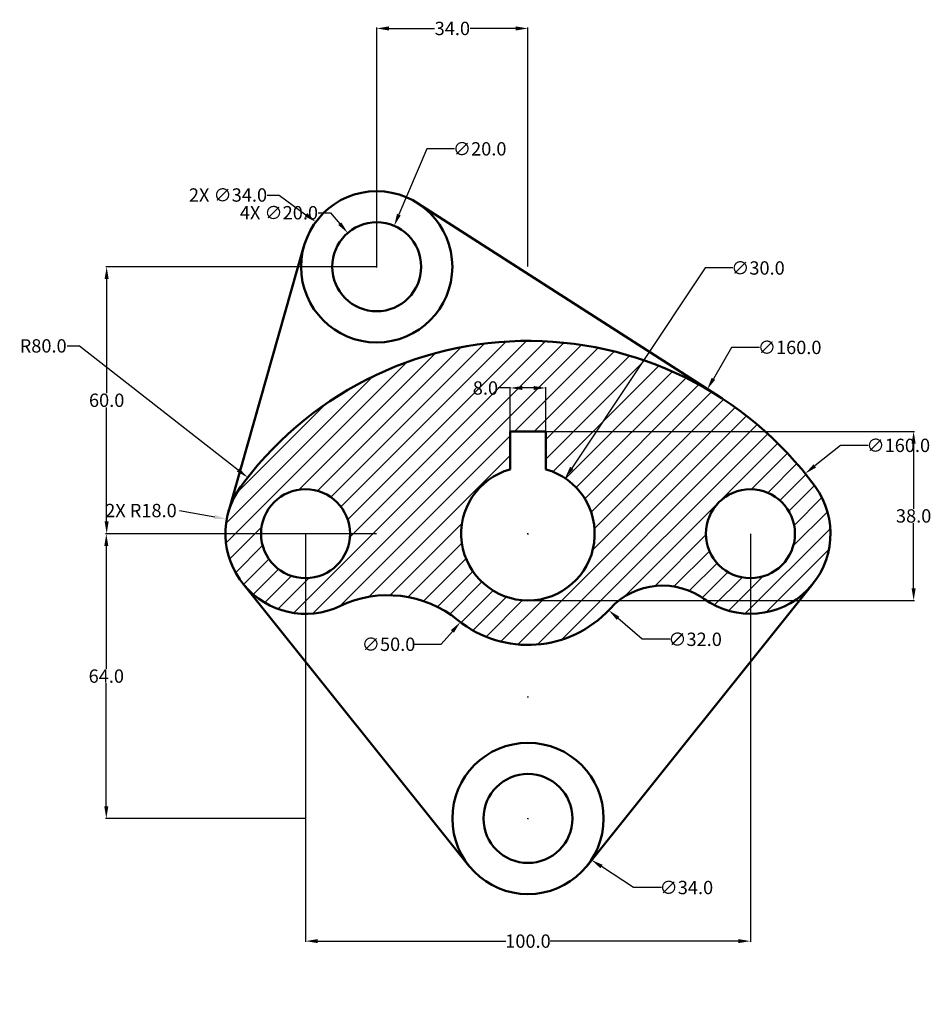
# Model space of a CAD drawing. Units: inches. Extents: x 315 to 520, y 214 to 435.
import ezdxf

# ---------------------------------------------------------------- set-up
doc = ezdxf.new("R2010")
doc.units = ezdxf.units.IN
doc.header["$MEASUREMENT"] = 0
for name, color, linetype, lineweight in [('M-DIMS', 2, 'Continuous', 25), ('M-HATC', 8, 'Continuous', 18), ('M-OUTL', 7, 'Continuous', 50)]:
    doc.layers.add(name, color=color, linetype=linetype, lineweight=lineweight)
doc.styles.get("Standard").update_dxf_attribs({"font": 'arial.ttf'})
doc.dimstyles.get("Standard").update_dxf_attribs({"dimtxt": 3, "dimasz": 2.75, "dimexe": 0.18, "dimexo": 0.0625, "dimgap": 0.09, "dimtad": 0, "dimtih": 1, "dimtoh": 1, "dimdec": 1, "dimzin": 0, "dimdsep": 46, "dimtxsty": 'Standard', "dimcen": 0.09, "dimadec": 0, "dimazin": 0, "dimtfac": 1, "dimtdec": 1, "dimtofl": 0, "dimtmove": 0, "dimatfit": 3, "dimfxl": 1, "dimtolj": 1, "dimtzin": 0, "dimarcsym": 0})

# ---------------------------------------------------------------- blocks, each defined once
blk = doc.blocks.new('*D1')
at = {"layer": 'Defpoints', "color": 0, "transparency": 16777216}
for p in [(379.7, 319.71), (479.7, 319.71), (479.7, 228.14)]:
    blk.add_point(p, dxfattribs=at)
at = {"layer": 'M-DIMS', "color": 0, "lineweight": -2, "transparency": 16777216}
for p, q in [((379.7, 319.65), (379.7, 227.96)), ((479.7, 319.65), (479.7, 227.96)), ((382.45, 228.14), (424.7, 228.14)), ((476.95, 228.14), (434.71, 228.14))]:
    blk.add_line(p, q, dxfattribs=at)
at = {"layer": 'M-DIMS', "color": 0, "transparency": 16777216}
for points in [[(382.45, 228.6), (382.45, 227.69), (379.7, 228.14)], [(476.95, 228.6), (476.95, 227.69), (479.7, 228.14)]]:
    blk.add_solid(points, dxfattribs=at)
at = {"layer": 'M-DIMS', "color": 0, "transparency": 16777216, "insert": (429.7, 228.14), "char_height": 3, "attachment_point": 5}
blk.add_mtext('\\A1;100.0', dxfattribs=at)
blk = doc.blocks.new('*D2')
at = {"layer": 'Defpoints', "color": 0, "transparency": 16777216}
for p in [(395.7, 379.71), (335, 319.71), (395.7, 319.71)]:
    blk.add_point(p, dxfattribs=at)
at = {"layer": 'M-DIMS', "color": 0, "lineweight": -2, "transparency": 16777216}
for p, q in [((395.64, 379.71), (334.82, 379.71)), ((335, 376.96), (335, 351.33)), ((335, 322.46), (335, 348.09)), ((395.64, 319.71), (334.82, 319.71))]:
    blk.add_line(p, q, dxfattribs=at)
at = {"layer": 'M-DIMS', "color": 0, "transparency": 16777216}
for points in [[(334.54, 376.96), (335.45, 376.96), (335, 379.71)], [(334.54, 322.46), (335.45, 322.46), (335, 319.71)]]:
    blk.add_solid(points, dxfattribs=at)
at = {"layer": 'M-DIMS', "color": 0, "transparency": 16777216, "insert": (335, 349.71), "char_height": 3, "attachment_point": 5}
blk.add_mtext('\\A1;60.0', dxfattribs=at)
blk = doc.blocks.new('*D3')
at = {"layer": 'Defpoints', "color": 0, "transparency": 16777216}
for p in [(379.7, 319.71), (334.92, 255.71), (379.7, 255.71)]:
    blk.add_point(p, dxfattribs=at)
at = {"layer": 'M-DIMS', "color": 0, "lineweight": -2, "transparency": 16777216}
for p, q in [((379.64, 319.71), (334.74, 319.71)), ((334.92, 316.96), (334.92, 289.33)), ((334.92, 258.46), (334.92, 286.09)), ((379.64, 255.71), (334.74, 255.71))]:
    blk.add_line(p, q, dxfattribs=at)
at = {"layer": 'M-DIMS', "color": 0, "transparency": 16777216}
for points in [[(334.46, 316.96), (335.38, 316.96), (334.92, 319.71)], [(334.46, 258.46), (335.38, 258.46), (334.92, 255.71)]]:
    blk.add_solid(points, dxfattribs=at)
at = {"layer": 'M-DIMS', "color": 0, "transparency": 16777216, "insert": (334.92, 287.71), "char_height": 3, "attachment_point": 5}
blk.add_mtext('\\A1;64.0', dxfattribs=at)
blk = doc.blocks.new('*D4')
at = {"layer": 'Defpoints', "color": 0, "transparency": 16777216}
for p in [(429.7, 433.28), (395.7, 379.71), (429.7, 379.71)]:
    blk.add_point(p, dxfattribs=at)
at = {"layer": 'M-DIMS', "color": 0, "lineweight": -2, "transparency": 16777216}
for p, q in [((395.7, 379.78), (395.7, 433.46)), ((398.45, 433.28), (408.72, 433.28)), ((426.95, 433.28), (416.68, 433.28)), ((429.7, 379.78), (429.7, 433.46))]:
    blk.add_line(p, q, dxfattribs=at)
at = {"layer": 'M-DIMS', "color": 0, "transparency": 16777216}
for points in [[(398.45, 433.74), (398.45, 432.82), (395.7, 433.28)], [(426.95, 433.74), (426.95, 432.82), (429.7, 433.28)]]:
    blk.add_solid(points, dxfattribs=at)
at = {"layer": 'M-DIMS', "color": 0, "transparency": 16777216, "insert": (412.7, 433.28), "char_height": 3, "attachment_point": 5}
blk.add_mtext('\\A1;34.0', dxfattribs=at)
blk = doc.blocks.new('*D5')
at = {"layer": 'Defpoints', "color": 0, "transparency": 16777216}
for p in [(415.47, 265.02), (443.93, 246.41)]:
    blk.add_point(p, dxfattribs=at)
at = {"layer": 'M-DIMS', "color": 0, "lineweight": -2, "transparency": 16777216}
for p, q in [((429.61, 255.71), (429.79, 255.71)), ((429.7, 255.62), (429.7, 255.8)), ((453.44, 240.19), (446.23, 244.91)), ((459.69, 240.19), (453.44, 240.19))]:
    blk.add_line(p, q, dxfattribs=at)
at = {"layer": 'M-DIMS', "color": 0, "transparency": 16777216}
blk.add_solid([(446.48, 245.29), (445.98, 244.52), (443.93, 246.41)], dxfattribs=at)
at = {"layer": 'M-DIMS', "color": 0, "transparency": 16777216, "insert": (465.3, 240.19), "char_height": 3, "attachment_point": 5}
blk.add_mtext('\\A1;∅34.0', dxfattribs=at)
blk = doc.blocks.new('*D6')
at = {"layer": 'Defpoints', "color": 0, "transparency": 16777216}
for p in [(399.62, 388.92), (391.79, 370.51)]:
    blk.add_point(p, dxfattribs=at)
at = {"layer": 'M-DIMS', "color": 0, "lineweight": -2, "transparency": 16777216}
for p, q in [((406.98, 406.22), (400.69, 391.45)), ((413.22, 406.22), (406.98, 406.22)), ((395.61, 379.71), (395.79, 379.71)), ((395.7, 379.62), (395.7, 379.8))]:
    blk.add_line(p, q, dxfattribs=at)
at = {"layer": 'M-DIMS', "color": 0, "transparency": 16777216}
blk.add_solid([(400.27, 391.63), (401.11, 391.27), (399.62, 388.92)], dxfattribs=at)
at = {"layer": 'M-DIMS', "color": 0, "transparency": 16777216, "insert": (418.84, 406.22), "char_height": 3, "attachment_point": 5}
blk.add_mtext('\\A1;∅20.0', dxfattribs=at)
blk = doc.blocks.new('*D7')
at = {"layer": 'Defpoints', "color": 0, "transparency": 16777216}
for p in [(469.99, 352.17), (389.41, 213.94)]:
    blk.add_point(p, dxfattribs=at)
at = {"layer": 'M-DIMS', "color": 0, "lineweight": -2, "transparency": 16777216}
for p, q in [((475.48, 361.59), (471.38, 354.54)), ((481.73, 361.59), (475.48, 361.59)), ((429.61, 283.05), (429.79, 283.05)), ((429.7, 282.96), (429.7, 283.14))]:
    blk.add_line(p, q, dxfattribs=at)
at = {"layer": 'M-DIMS', "color": 0, "transparency": 16777216}
blk.add_solid([(470.98, 354.77), (471.77, 354.31), (469.99, 352.17)], dxfattribs=at)
at = {"layer": 'M-DIMS', "color": 0, "transparency": 16777216, "insert": (488.51, 361.59), "char_height": 3, "attachment_point": 5}
blk.add_mtext('\\A1;∅160.0', dxfattribs=at)
blk = doc.blocks.new('*D8')
at = {"layer": 'Defpoints', "color": 0, "transparency": 16777216}
for p in [(438.02, 332.19), (421.38, 307.23)]:
    blk.add_point(p, dxfattribs=at)
at = {"layer": 'M-DIMS', "color": 0, "lineweight": -2, "transparency": 16777216}
for p, q in [((469.53, 379.44), (439.55, 334.48)), ((475.77, 379.44), (469.53, 379.44)), ((429.61, 319.71), (429.79, 319.71)), ((429.7, 319.62), (429.7, 319.8))]:
    blk.add_line(p, q, dxfattribs=at)
at = {"layer": 'M-DIMS', "color": 0, "transparency": 16777216}
blk.add_solid([(439.17, 334.74), (439.93, 334.23), (438.02, 332.19)], dxfattribs=at)
at = {"layer": 'M-DIMS', "color": 0, "transparency": 16777216, "insert": (481.39, 379.44), "char_height": 3, "attachment_point": 5}
blk.add_mtext('\\A1;∅30.0', dxfattribs=at)
blk = doc.blocks.new('*D9')
at = {"layer": 'Defpoints', "color": 0, "transparency": 16777216}
for p in [(492.02, 333.22), (367.39, 232.89)]:
    blk.add_point(p, dxfattribs=at)
at = {"layer": 'M-DIMS', "color": 0, "lineweight": -2, "transparency": 16777216}
for p, q in [((499.91, 339.57), (494.16, 334.94)), ((506.15, 339.57), (499.91, 339.57)), ((429.61, 283.05), (429.79, 283.05)), ((429.7, 282.96), (429.7, 283.14))]:
    blk.add_line(p, q, dxfattribs=at)
at = {"layer": 'M-DIMS', "color": 0, "transparency": 16777216}
blk.add_solid([(493.87, 335.3), (494.45, 334.59), (492.02, 333.22)], dxfattribs=at)
at = {"layer": 'M-DIMS', "color": 0, "transparency": 16777216, "insert": (512.93, 339.57), "char_height": 3, "attachment_point": 5}
blk.add_mtext('\\A1;∅160.0', dxfattribs=at)
blk = doc.blocks.new('*D10')
at = {"layer": 'Defpoints', "color": 0, "transparency": 16777216}
for p in [(447.85, 302.51), (472.05, 281.57)]:
    blk.add_point(p, dxfattribs=at)
at = {"layer": 'M-DIMS', "color": 0, "lineweight": -2, "transparency": 16777216}
for p, q in [((455.4, 295.98), (449.93, 300.71)), ((461.65, 295.98), (455.4, 295.98))]:
    blk.add_line(p, q, dxfattribs=at)
blk.add_arc((459.95, 292.04), 16, 137.7686, 139.78, dxfattribs=at)
at = {"layer": 'M-DIMS', "color": 0, "transparency": 16777216}
blk.add_solid([(450.23, 301.05), (449.63, 300.36), (447.85, 302.51)], dxfattribs=at)
at = {"layer": 'M-DIMS', "color": 0, "transparency": 16777216, "insert": (467.26, 295.98), "char_height": 3, "attachment_point": 5}
blk.add_mtext('\\A1;∅32.0', dxfattribs=at)
blk = doc.blocks.new('*D11')
at = {"layer": 'Defpoints', "color": 0, "transparency": 16777216}
for p in [(414.5, 299.84), (381.88, 261.94)]:
    blk.add_point(p, dxfattribs=at)
at = {"layer": 'M-DIMS', "color": 0, "lineweight": -2, "transparency": 16777216}
for p, q in [((410.22, 294.86), (412.71, 297.75)), ((403.97, 294.86), (410.22, 294.86))]:
    blk.add_line(p, q, dxfattribs=at)
blk.add_arc((398.19, 280.89), 25, 48.8679, 50.7919, dxfattribs=at)
at = {"layer": 'M-DIMS', "color": 0, "transparency": 16777216}
blk.add_solid([(412.36, 298.05), (413.05, 297.46), (414.5, 299.84)], dxfattribs=at)
at = {"layer": 'M-DIMS', "color": 0, "transparency": 16777216, "insert": (398.36, 294.86), "char_height": 3, "attachment_point": 5}
blk.add_mtext('\\A1;∅50.0', dxfattribs=at)
blk = doc.blocks.new('*D12')
at = {"layer": 'Defpoints', "color": 0, "transparency": 16777216}
for p in [(425.7, 352.47), (425.7, 342.71), (433.7, 342.71)]:
    blk.add_point(p, dxfattribs=at)
at = {"layer": 'M-DIMS', "color": 0, "lineweight": -2, "transparency": 16777216}
for p, q in [((425.7, 352.47), (422.95, 352.47)), ((425.7, 342.78), (425.7, 352.65)), ((430.95, 352.47), (428.45, 352.47)), ((433.7, 342.78), (433.7, 352.65))]:
    blk.add_line(p, q, dxfattribs=at)
at = {"layer": 'M-DIMS', "color": 0, "transparency": 16777216}
for points in [[(428.45, 352.92), (428.45, 352.01), (425.7, 352.47)], [(430.95, 352.92), (430.95, 352.01), (433.7, 352.47)]]:
    blk.add_solid(points, dxfattribs=at)
at = {"layer": 'M-DIMS', "color": 0, "transparency": 16777216, "insert": (420.13, 352.47), "char_height": 3, "attachment_point": 5}
blk.add_mtext('\\A1;8.0', dxfattribs=at)
blk = doc.blocks.new('*D13')
at = {"layer": 'Defpoints', "color": 0, "transparency": 16777216}
for p in [(429.7, 342.71), (516.38, 342.71), (429.7, 304.71)]:
    blk.add_point(p, dxfattribs=at)
at = {"layer": 'M-DIMS', "color": 0, "lineweight": -2, "transparency": 16777216}
for p, q in [((429.76, 342.71), (516.56, 342.71)), ((516.38, 339.96), (516.38, 325.34)), ((516.38, 307.46), (516.38, 322.09)), ((429.76, 304.71), (516.56, 304.71))]:
    blk.add_line(p, q, dxfattribs=at)
at = {"layer": 'M-DIMS', "color": 0, "transparency": 16777216}
for points in [[(515.92, 339.96), (516.84, 339.96), (516.38, 342.71)], [(515.92, 307.46), (516.84, 307.46), (516.38, 304.71)]]:
    blk.add_solid(points, dxfattribs=at)
at = {"layer": 'M-DIMS', "color": 0, "transparency": 16777216, "insert": (516.38, 323.71), "char_height": 3, "attachment_point": 5}
blk.add_mtext('\\A1;38.0', dxfattribs=at)
blk = doc.blocks.new('BRACKET-MOUNTING-EYE')
for radius in [17, 10]:
    blk.add_circle((0, 0), radius)
blk = doc.blocks.new('*D15')
at = {"layer": 'Defpoints', "color": 0, "transparency": 16777216}
for p in [(366.7, 332.35), (429.7, 283.05)]:
    blk.add_point(p, dxfattribs=at)
at = {"layer": 'M-DIMS', "color": 0, "lineweight": -2, "transparency": 16777216}
for p, q in [((326.14, 361.93), (328.89, 361.93)), ((328.89, 361.93), (364.53, 334.05)), ((429.61, 283.05), (429.79, 283.05)), ((429.7, 282.96), (429.7, 283.14))]:
    blk.add_line(p, q, dxfattribs=at)
at = {"layer": 'M-DIMS', "color": 0, "transparency": 16777216}
blk.add_solid([(364.81, 334.41), (364.25, 333.69), (366.7, 332.35)], dxfattribs=at)
at = {"layer": 'M-DIMS', "color": 0, "transparency": 16777216, "insert": (320.73, 361.93), "char_height": 3, "attachment_point": 5}
blk.add_mtext('\\A1;R80.0', dxfattribs=at)
blk = doc.blocks.new('*D16')
at = {"layer": 'Defpoints', "color": 0, "transparency": 16777216}
for p in [(362, 322.97), (379.7, 319.71)]:
    blk.add_point(p, dxfattribs=at)
at = {"layer": 'M-DIMS', "color": 0, "lineweight": -2, "transparency": 16777216}
for p, q in [((351.38, 324.92), (359.29, 323.47)), ((379.61, 319.71), (379.79, 319.71)), ((379.7, 319.62), (379.7, 319.8))]:
    blk.add_line(p, q, dxfattribs=at)
at = {"layer": 'M-DIMS', "color": 0, "transparency": 16777216}
blk.add_solid([(359.38, 323.92), (359.21, 323.02), (362, 322.97)], dxfattribs=at)
at = {"layer": 'M-DIMS', "color": 0, "transparency": 16777216, "insert": (342.71, 324.92), "char_height": 3, "attachment_point": 5}
blk.add_mtext('\\A1;2X R18.0', dxfattribs=at)
blk = doc.blocks.new('*D17')
at = {"layer": 'Defpoints', "color": 0, "transparency": 16777216}
for p in [(382.01, 389.79), (409.39, 369.63)]:
    blk.add_point(p, dxfattribs=at)
at = {"layer": 'M-DIMS', "color": 0, "lineweight": -2, "transparency": 16777216}
for p, q in [((371.05, 395.84), (373.8, 395.84)), ((373.8, 395.84), (379.8, 391.42)), ((395.61, 379.71), (395.79, 379.71)), ((395.7, 379.62), (395.7, 379.8))]:
    blk.add_line(p, q, dxfattribs=at)
at = {"layer": 'M-DIMS', "color": 0, "transparency": 16777216}
blk.add_solid([(380.07, 391.79), (379.53, 391.05), (382.01, 389.79)], dxfattribs=at)
at = {"layer": 'M-DIMS', "color": 0, "transparency": 16777216, "insert": (362.27, 395.84), "char_height": 3, "attachment_point": 5}
blk.add_mtext('\\A1;2X ∅34.0', dxfattribs=at)
blk = doc.blocks.new('*D18')
at = {"layer": 'Defpoints', "color": 0, "transparency": 16777216}
for p in [(389.19, 387.31), (402.21, 372.12)]:
    blk.add_point(p, dxfattribs=at)
at = {"layer": 'M-DIMS', "color": 0, "lineweight": -2, "transparency": 16777216}
for p, q in [((382.54, 391.86), (385.29, 391.86)), ((385.29, 391.86), (387.41, 389.39)), ((395.61, 379.71), (395.79, 379.71)), ((395.7, 379.62), (395.7, 379.8))]:
    blk.add_line(p, q, dxfattribs=at)
at = {"layer": 'M-DIMS', "color": 0, "transparency": 16777216}
blk.add_solid([(387.75, 389.69), (387.06, 389.1), (389.19, 387.31)], dxfattribs=at)
at = {"layer": 'M-DIMS', "color": 0, "transparency": 16777216, "insert": (373.72, 391.86), "char_height": 3, "attachment_point": 5}
blk.add_mtext('\\A1;4X ∅20.0', dxfattribs=at)

msp = doc.modelspace()

# ---------------------------------------------------------------- hatches: boundary and pattern name
at = {"layer": 'M-HATC'}
h = msp.add_hatch(dxfattribs=at)
h.set_pattern_fill('ANSI31', color=256, scale=25)
h.paths.add_polyline_path([(365.19, 330.36, 0.779298), (387.44, 303.46, -0.289261), (413.95, 300.3, 0.396987), (448.15, 302.84, -0.379152), (469.25, 305.06, 0.852286), (494.22, 330.36, 0.506788)])
h.paths.add_polyline_path([(489.7, 319.71, -1), (469.7, 319.71, -1)], flags=16)
h.paths.add_polyline_path([(425.7, 334.17), (425.7, 342.71), (433.7, 342.71), (433.7, 334.17, -7.364208)], flags=16)
h.paths.add_polyline_path([(389.7, 319.71, -1), (369.7, 319.71, -1)], flags=16)
h.paths.add_polyline_path([(416.49, 349.35), (423.81, 349.35), (423.81, 355.53), (416.49, 355.53)], flags=24)

# ---------------------------------------------------------------- linework, layer by layer
at = {"layer": 'M-OUTL'}
for p, q in [((404.88, 394.02), (472.9, 350.39)), ((379.35, 384.36), (362.39, 324.63)), ((425.7, 334.17), (425.7, 342.71)), ((433.7, 342.71), (425.7, 342.71)), ((433.7, 334.17), (433.7, 342.71)), ((416.44, 245.08), (365.65, 308.46)), ((442.97, 245.08), (493.75, 308.46)), ((469.75, 304.71), (469.72, 304.71))]:
    msp.add_line(p, q, dxfattribs=at)
for centre in [(379.7, 319.71), (479.7, 319.71)]:
    msp.add_circle(centre, 10, dxfattribs=at)
for centre, radius, start, end in [((429.7, 283.05), 80, 36.2493, 146.2127), ((429.7, 319.71), 15, 105.466, 74.534), ((379.7, 319.71), 18, 143.7507, 295.4676), ((479.7, 319.71), 18, 234.4874, 36.2493), ((459.95, 292.04), 16, 52.3938, 137.5448), ((398.19, 280.89), 25, 50.9351, 115.4676), ((429.7, 319.71), 25, 230.9351, 317.5448)]:
    msp.add_arc(centre, radius, start, end, dxfattribs=at)

# ---------------------------------------------------------------- block references
for p in [(395.7, 379.71), (429.7, 255.71)]:
    msp.add_blockref('BRACKET-MOUNTING-EYE', p, dxfattribs=at)

# ---------------------------------------------------------------- dimensions: what is measured, and where the dimension line sits
at = {"layer": 'M-DIMS'}
for base, p1, p2, picture, middle in [((429.7, 433.28), (395.7, 379.71), (429.7, 379.71), '*D4', (412.7, 433.28)), ((425.7, 352.47), (433.7, 342.71), (425.7, 342.71), '*D12', (420.13, 352.47)), ((479.7, 228.14), (379.7, 319.71), (479.7, 319.71), '*D1', (429.7, 228.14))]:
    dim = msp.add_linear_dim(base=base, p1=p1, p2=p2, dimstyle='Standard', override={"dimclrd": 0, "dimclre": 0, "dimclrt": 0}, dxfattribs=at)
    dim.commit()
    dim.dimension.update_dxf_attribs({"geometry": picture, "text_midpoint": middle})
for p1, p2, picture, middle in [((391.79, 370.51), (399.62, 388.92), '*D6', (418.84, 406.22)), ((421.38, 307.23), (438.02, 332.19), '*D8', (481.39, 379.44)), ((389.41, 213.94), (469.99, 352.17), '*D7', (488.51, 361.59)), ((367.39, 232.89), (492.02, 333.22), '*D9', (512.93, 339.57)), ((472.05, 281.57), (447.85, 302.51), '*D10', (467.26, 295.98)), ((381.88, 261.94), (414.5, 299.84), '*D11', (398.36, 294.86)), ((415.47, 265.02), (443.93, 246.41), '*D5', (465.3, 240.19))]:
    dim = msp.add_diameter_dim_2p(p1=p1, p2=p2, dimstyle='Standard', override={"dimclrd": 0, "dimclre": 0, "dimclrt": 0}, dxfattribs=at)
    dim.commit()
    dim.dimension.update_dxf_attribs({"geometry": picture, "text_midpoint": middle, "dimtype": 163})
for p1, p2, text, picture, middle in [((409.39, 369.63), (382.01, 389.79), '2X <>', '*D17', (362.27, 395.84)), ((402.21, 372.12), (389.19, 387.31), '4X <>', '*D18', (373.72, 391.86))]:
    dim = msp.add_diameter_dim_2p(p1=p1, p2=p2, text=text, dimstyle='Standard', override={"dimdec": 1, "dimlfac": 1, "dimrnd": 0, "dimzin": 0, "dimdsep": 46, "dimlunit": 2}, dxfattribs=at)
    dim.commit()
    dim.dimension.update_dxf_attribs({"geometry": picture, "text_midpoint": middle, "dimtype": 163})
for base, p1, p2, picture, middle in [((335, 319.71), (395.7, 379.71), (395.7, 319.71), '*D2', (335, 349.71)), ((516.38, 342.71), (429.7, 304.71), (429.7, 342.71), '*D13', (516.38, 323.71)), ((334.92, 255.71), (379.7, 319.71), (379.7, 255.71), '*D3', (334.92, 287.71))]:
    dim = msp.add_linear_dim(base=base, p1=p1, p2=p2, angle=90, dimstyle='Standard', override={"dimclrd": 0, "dimclre": 0, "dimclrt": 0}, dxfattribs=at)
    dim.commit()
    dim.dimension.update_dxf_attribs({"geometry": picture, "text_midpoint": middle})
dim = msp.add_radius_dim(center=(429.7, 283.05), mpoint=(366.7, 332.35), dimstyle='Standard', override={"dimdec": 1, "dimlfac": 1, "dimrnd": 0, "dimzin": 0, "dimdsep": 46, "dimlunit": 2}, dxfattribs=at)
dim.commit()
dim.dimension.update_dxf_attribs({"geometry": '*D15', "text_midpoint": (320.73, 361.93), "dimtype": 164})
dim = msp.add_radius_dim(center=(379.7, 319.71), mpoint=(362, 322.97), text='2X <>', dimstyle='Standard', override={"dimdec": 1, "dimlfac": 1, "dimrnd": 0, "dimzin": 0, "dimdsep": 46, "dimlunit": 2}, dxfattribs=at)
dim.commit()
dim.dimension.update_dxf_attribs({"geometry": '*D16', "text_midpoint": (351.38, 324.92), "dimtype": 164})

doc.saveas('drawing.dxf')
